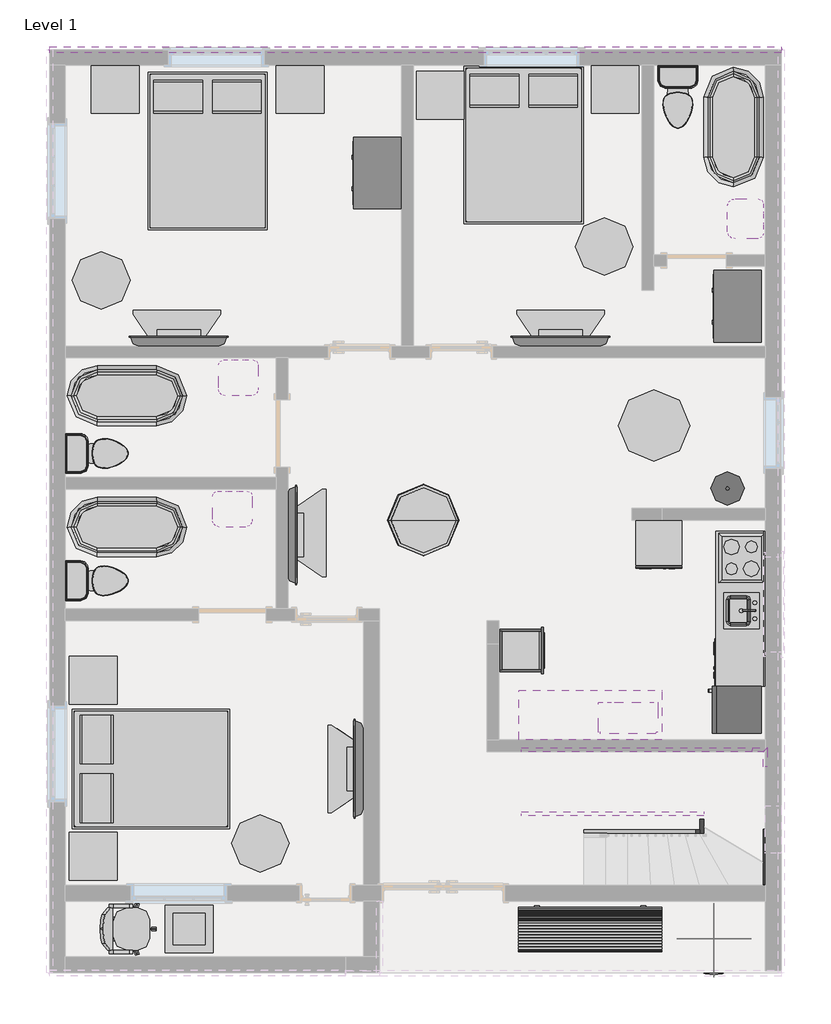
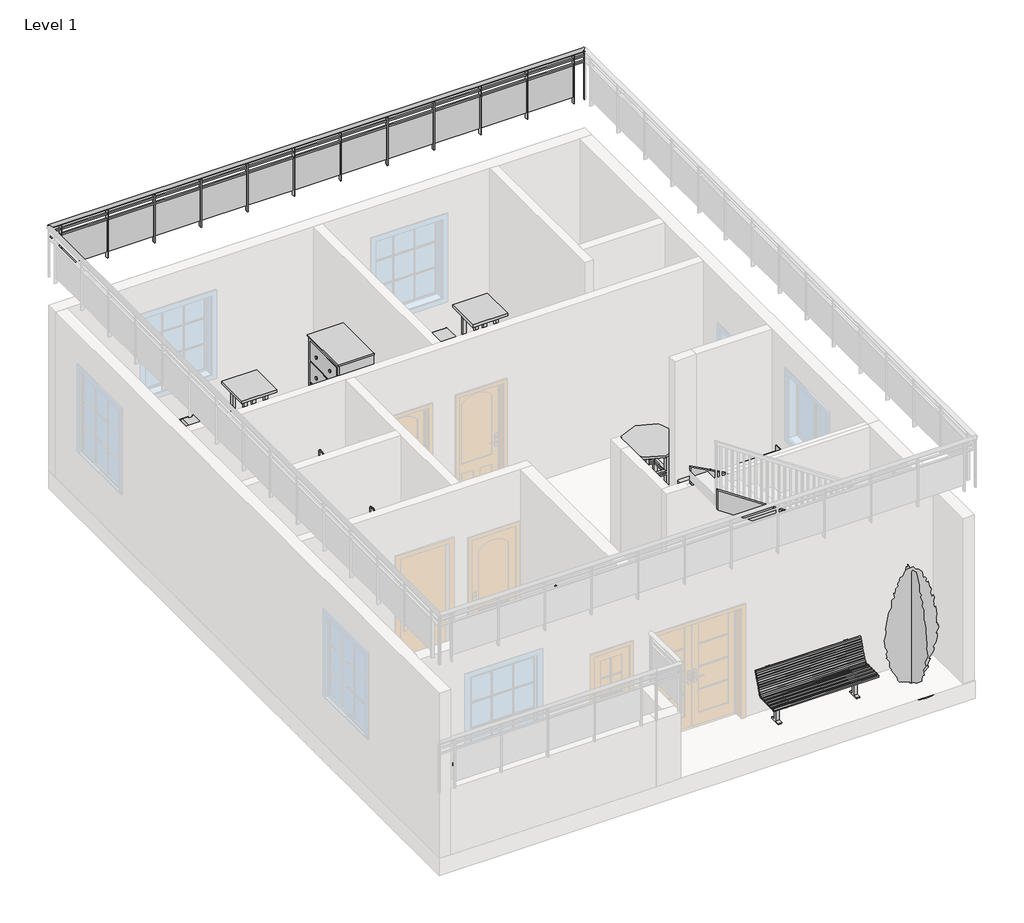
# One storey, part 4 of 4: 28 furniture elements, 11 flow terminals, 10 members, 7 proxies, 2 geographic elements, 1 railing.
"""IFC4 building model written with IfcOpenShell, lengths in millimetres."""

from ifc_helpers import new_model, si_unit, point, frame, origin, place, context, project, spatial, polyline, ellipse_curve, trimmed, outline, extrude, transform, mapped, element, save
from ifc_brep_helpers import plane_surface, extruded_surface, advanced_brep
from components import proxy_a6faaae8, proxy_53e5fb40, proxy_45b28599, kitchenette_medium_kitchenette_medium_844211aa, proxy_8a8d5ab2, proxy_8b8c2dc4, proxy_c523a7b7, flow_terminal_871c2e40, flow_terminal_d49f872f, flow_terminal_62a433f7, toilet_domestic_3d_toilet_domestic_3d_f7549cf7, toilet_domestic_3d_toilet_domestic_3d_183bbd19, flow_terminal_b374fae2, furniture_1d2926bd, chair_executive_chair_executive_8d69e98c, furniture_c6510c7c, furniture_1447f48d, furniture_33655958, furniture_fdf74506, tv_stand_tv_stand_6ce107e5, furniture_b5c51a22, furniture_905aceb5, furniture_b2396e53, furniture_5bc9ed15, furniture_c80d6d9c, geographic_element_235d1464, rpc_tree_conifer_chinese_juniper_7_1b9786cd

model = new_model("IFC4")

# Units and contexts
model_context = context("Model", 3, world=origin())
ifc_project = project(units=[si_unit("LENGTHUNIT", "METRE", prefix="MILLI")], contexts=[model_context])

# Site, building, storey
site = spatial("IfcSite", under=ifc_project)
building = spatial("IfcBuilding", under=site)
storey = spatial("IfcBuildingStorey", under=building, Name="Level 1", Elevation=0.0)

# Proxies
placement = place(None, origin())
proxy_shape = proxy_a6faaae8(model_context)
element("IfcBuildingElementProxy", 1, Name="Cook Top-4 Unit2 : 22\" x 20\"", ObjectType="Cook Top-4 Unit2 : 22\" x 20\"", at=placement, inside=storey, context=model_context, shape_type="MappedRepresentation", body=[
    mapped(proxy_shape, transform((5037.4355823, 3615.7840324, 0.0), x_axis=(0.0, -1.0000000000000002, 0.0), y_axis=(1.0000000000000002, 0.0, 0.0), z_axis=(0.0, 0.0, 1.0))),
])
proxy_2_shape = proxy_53e5fb40(model_context)
element("IfcBuildingElementProxy", 2, Name="Dishwasher : 23\" x 23 11/16\" x 33 1/2\"", ObjectType="Dishwasher : 23\" x 23 11/16\" x 33 1/2\"", at=placement, inside=storey, context=model_context, shape_type="MappedRepresentation", body=[
    mapped(proxy_2_shape, transform((3613.7181138, 3535.0719677, 0.0), x_axis=(1.0000000000000002, 0.0, 0.0), y_axis=(0.0, 1.0000000000000002, 0.0), z_axis=(0.0, 0.0, 1.0))),
])
proxy_3_shape = proxy_45b28599(model_context)
element("IfcBuildingElementProxy", 3, Name="Dishwasher : 24\" x 24\" x 34\"", ObjectType="Dishwasher : 24\" x 24\" x 34\"", at=placement, inside=storey, context=model_context, shape_type="MappedRepresentation", body=[
    mapped(proxy_3_shape, transform((4745.5860175, 2664.6015009, 0.0), x_axis=(0.0, -1.0000000000000002, 0.0), y_axis=(1.0000000000000002, 0.0, 0.0), z_axis=(0.0, 0.0, 1.0))),
])
kitchenette_medium_kitchenette_medium_shape = kitchenette_medium_kitchenette_medium_844211aa(model_context)
element("IfcBuildingElementProxy", 4, Name="Kitchenette - Medium : Kitchenette - Medium", ObjectType="Kitchenette - Medium : Kitchenette - Medium", at=placement, inside=storey, context=model_context, shape_type="MappedRepresentation", body=[
    mapped(kitchenette_medium_kitchenette_medium_shape, transform((5342.2355823, 3291.6217374, 0.0), x_axis=(0.0, -1.0000000000000002, 0.0), y_axis=(1.0000000000000002, 0.0, 0.0), z_axis=(0.0, 0.0, 1.0))),
])
proxy_4_shape = proxy_8a8d5ab2(model_context)
element("IfcBuildingElementProxy", 5, Name="Microwave : 30\" x 16\" x 18\"", ObjectType="Microwave : 30\" x 16\" x 18\"", at=placement, inside=storey, context=model_context, shape_type="MappedRepresentation", body=[
    mapped(proxy_4_shape, transform((4089.9284596, 1218.0035266, 609.6), x_axis=(-1.0000000000000004, 0.0, 0.0), y_axis=(0.0, -1.0000000000000004, 0.0), z_axis=(0.0, 0.0, 1.0))),
])
proxy_5_shape = proxy_8b8c2dc4(model_context)
element("IfcBuildingElementProxy", 6, Name="Oven Double-Built-in : 21 1/2\" x 39 1/4\" x 21\"", ObjectType="Oven Double-Built-in : 21 1/2\" x 39 1/4\" x 21\"", at=placement, inside=storey, context=model_context, shape_type="MappedRepresentation", body=[
    mapped(proxy_5_shape, transform((2359.1014412, 2469.8589597, 0.0), x_axis=(0.0, 1.0000000000000002, 0.0), y_axis=(-1.0000000000000002, 0.0, 0.0), z_axis=(0.0, 0.0, 1.0))),
])
proxy_6_shape = proxy_c523a7b7(model_context)
element("IfcBuildingElementProxy", 7, Name="Refrigerator : 24\" x 25\" LH", ObjectType="Refrigerator : 24\" x 25\" LH", at=placement, inside=storey, context=model_context, shape_type="MappedRepresentation", body=[
    mapped(proxy_6_shape, transform((4991.7866108, 1679.0340324, 0.0), x_axis=(0.0, -1.0000000000000002, 0.0), y_axis=(1.0000000000000002, 0.0, 0.0), z_axis=(0.0, 0.0, 1.0))),
])

# Flow terminals
flow_terminal_shape = flow_terminal_871c2e40(model_context)
element("IfcFlowTerminal", 8, ObjectType="Sink Kitchen-Island : 18\" x 18\"", at=placement, inside=storey, context=model_context, shape_type="MappedRepresentation", body=[
    mapped(flow_terminal_shape, transform((5035.0901812, 2958.373273, -14.4), x_axis=(0.0, -1.0000000000000002, 0.0), y_axis=(1.0000000000000002, 0.0, 0.0), z_axis=(0.0, 0.0, 1.0))),
])
flow_terminal_2_shape = flow_terminal_d49f872f(model_context)
element("IfcFlowTerminal", 9, ObjectType="Sink Vanity-Round : 19\" x 19\"", at=placement, inside=storey, context=model_context, shape_type="MappedRepresentation", body=[
    mapped(flow_terminal_2_shape, transform((4956.2873228, 4587.4155119, 609.6), x_axis=(-1.0000000000000004, 0.0, 0.0), y_axis=(0.0, -1.0000000000000004, 0.0), z_axis=(0.0, 0.0, 1.0))),
])
flow_terminal_3_shape = flow_terminal_62a433f7(model_context)
element("IfcFlowTerminal", 10, ObjectType="Sink Vanity-Square : 20\" x 18\"", at=placement, inside=storey, context=model_context, shape_type="MappedRepresentation", body=[
    mapped(flow_terminal_3_shape, transform((-1404.4536583, 5962.9386313, 914.4), x_axis=(1.0, 0.0, 0.0), y_axis=(0.0, 1.0, 0.0), z_axis=(0.0, 0.0, 1.0))),
])
element("IfcFlowTerminal", 11, ObjectType="Sink Vanity-Square : 20\" x 18\"", at=placement, inside=storey, context=model_context, shape_type="MappedRepresentation", body=[
    mapped(flow_terminal_3_shape, transform((-1480.6536583, 4286.5386313, 914.4), x_axis=(1.0, 0.0, 0.0), y_axis=(0.0, 1.0, 0.0), z_axis=(0.0, 0.0, 1.0))),
])
element("IfcFlowTerminal", 12, ObjectType="Sink Vanity-Square : 20\" x 18\"", at=placement, inside=storey, context=model_context, shape_type="MappedRepresentation", body=[
    mapped(flow_terminal_3_shape, transform((5136.6901812, 7962.173273, 914.4), x_axis=(0.0, -1.0, 0.0), y_axis=(1.0, 0.0, 0.0), z_axis=(0.0, 0.0, 1.0))),
])
toilet_domestic_3d_toilet_domestic_3d_shape = toilet_domestic_3d_toilet_domestic_3d_f7549cf7(model_context)
toilet_domestic_3d_toilet_domestic_3d_2_shape = toilet_domestic_3d_toilet_domestic_3d_183bbd19(model_context)
element("IfcFlowTerminal", 13, ObjectType="Toilet-Domestic-3D : Toilet-Domestic-3D", at=placement, inside=storey, context=model_context, shape_type="MappedRepresentation", body=[
    mapped(toilet_domestic_3d_toilet_domestic_3d_shape, transform((-3103.8683904, 4949.2840324, 0.0), x_axis=(0.0, 1.0000000000000002, 0.0), y_axis=(-1.0000000000000002, 0.0, 0.0), z_axis=(0.0, 0.0, 1.0))),
    mapped(toilet_domestic_3d_toilet_domestic_3d_2_shape, transform((-3103.8683904, 4949.2840324, 0.0), x_axis=(0.0, 1.0000000000000002, 0.0), y_axis=(-1.0000000000000002, 0.0, 0.0), z_axis=(0.0, 0.0, 1.0))),
])
element("IfcFlowTerminal", 14, ObjectType="Toilet-Domestic-3D : Toilet-Domestic-3D", at=placement, inside=storey, context=model_context, shape_type="MappedRepresentation", body=[
    mapped(toilet_domestic_3d_toilet_domestic_3d_shape, transform((-3103.8683904, 3323.6840324, 0.0), x_axis=(0.0, 1.0000000000000002, 0.0), y_axis=(-1.0000000000000002, 0.0, 0.0), z_axis=(0.0, 0.0, 1.0))),
    mapped(toilet_domestic_3d_toilet_domestic_3d_2_shape, transform((-3103.8683904, 3323.6840324, 0.0), x_axis=(0.0, 1.0000000000000002, 0.0), y_axis=(-1.0000000000000002, 0.0, 0.0), z_axis=(0.0, 0.0, 1.0))),
])
element("IfcFlowTerminal", 15, ObjectType="Toilet-Domestic-3D : Toilet-Domestic-3D", at=placement, inside=storey, context=model_context, shape_type="MappedRepresentation", body=[
    mapped(toilet_domestic_3d_toilet_domestic_3d_shape, transform((4224.6355823, 9407.5880051, 0.0), x_axis=(1.0, 0.0, 0.0), y_axis=(0.0, 1.0, 0.0), z_axis=(0.0, 0.0, 1.0))),
    mapped(toilet_domestic_3d_toilet_domestic_3d_2_shape, transform((4224.6355823, 9407.5880051, 0.0), x_axis=(1.0, 0.0, 0.0), y_axis=(0.0, 1.0, 0.0), z_axis=(0.0, 0.0, 1.0))),
])
flow_terminal_4_shape = flow_terminal_b374fae2(model_context)
element("IfcFlowTerminal", 16, ObjectType="Tub-Free Standing-3D : 30\" x 60\"", at=placement, inside=storey, context=model_context, shape_type="MappedRepresentation", body=[
    mapped(flow_terminal_4_shape, transform((-2811.1644177, 4009.4840324, 0.0), x_axis=(0.0, 1.0000000000000002, 0.0), y_axis=(-1.0000000000000002, 0.0, 0.0), z_axis=(0.0, 0.0, 1.0))),
])
element("IfcFlowTerminal", 17, ObjectType="Tub-Free Standing-3D : 30\" x 60\"", at=placement, inside=storey, context=model_context, shape_type="MappedRepresentation", body=[
    mapped(flow_terminal_4_shape, transform((-2811.1644177, 5685.8840324, 0.0), x_axis=(0.0, 1.0000000000000002, 0.0), y_axis=(-1.0000000000000002, 0.0, 0.0), z_axis=(0.0, 0.0, 1.0))),
])
element("IfcFlowTerminal", 18, ObjectType="Tub-Free Standing-3D : 30\" x 60\"", at=placement, inside=storey, context=model_context, shape_type="MappedRepresentation", body=[
    mapped(flow_terminal_4_shape, transform((4935.8355823, 9114.8840324, 0.0), x_axis=(1.0000000000000007, 0.0, 0.0), y_axis=(0.0, 1.0000000000000007, 0.0), z_axis=(0.0, 0.0, 1.0))),
])

# Furniture
furniture_shape = furniture_1d2926bd(model_context)
element("IfcFurniture", 19, ObjectType="Bed-Box : Queen 60\" x 79\"", at=placement, inside=storey, context=model_context, shape_type="MappedRepresentation", body=[
    mapped(furniture_shape, transform((-2740.7939259, 584.2315734, 0.0), x_axis=(0.0, 1.0000000000000002, 0.0), y_axis=(-1.0000000000000002, 0.0, 0.0), z_axis=(0.0, 0.0, 1.0))),
])
element("IfcFurniture", 20, ObjectType="Bed-Box : Queen 60\" x 79\"", at=placement, inside=storey, context=model_context, shape_type="MappedRepresentation", body=[
    mapped(furniture_shape, transform((-2121.6168767, 9044.5135406, 0.0), x_axis=(1.0000000000000002, 0.0, 0.0), y_axis=(0.0, 1.0000000000000002, 0.0), z_axis=(0.0, 0.0, 1.0))),
])
element("IfcFurniture", 21, ObjectType="Bed-Box : Queen 60\" x 79\"", at=placement, inside=storey, context=model_context, shape_type="MappedRepresentation", body=[
    mapped(furniture_shape, transform((1916.9831233, 9120.7135406, 0.0), x_axis=(1.0, 0.0, 0.0), y_axis=(0.0, 1.0, 0.0), z_axis=(0.0, 0.0, 1.0))),
])
chair_executive_chair_executive_shape = chair_executive_chair_executive_8d69e98c(model_context)
element("IfcFurniture", 22, ObjectType="Chair-Executive : Chair-Executive", at=placement, inside=storey, context=model_context, shape_type="MappedRepresentation", body=[
    mapped(chair_executive_chair_executive_shape, transform((-2804.7103194, -980.3251479, 0.0), x_axis=(0.0, -1.0000000000000004, 0.0), y_axis=(1.0000000000000004, 0.0, 0.0), z_axis=(0.0, 0.0, 1.0))),
])
furniture_2_shape = furniture_c6510c7c(model_context)
element("IfcFurniture", 23, ObjectType="Counter Top w Sink Hole : 24\" Depth", at=placement, inside=storey, context=model_context, shape_type="MappedRepresentation", body=[
    mapped(furniture_2_shape, transform((5342.2355823, 2758.2217374, -14.4), x_axis=(0.0, -1.0000000000000002, 0.0), y_axis=(1.0000000000000002, 0.0, 0.0), z_axis=(0.0, 0.0, 1.0))),
])
furniture_3_shape = furniture_1447f48d(model_context)
element("IfcFurniture", 24, ObjectType="Counter Top w Sink Hole : 24\" Depth", at=placement, inside=storey, context=model_context, shape_type="MappedRepresentation", body=[
    mapped(furniture_3_shape, transform((3393.0978774, 1926.6840324, 609.6), x_axis=(1.0, 0.0, 0.0), y_axis=(0.0, 1.0, 0.0), z_axis=(0.0, 0.0, 1.0))),
])
furniture_4_shape = furniture_33655958(model_context)
element("IfcFurniture", 25, ObjectType="Dresser : 48\" x 72\" x 24\"", at=placement, inside=storey, context=model_context, shape_type="MappedRepresentation", body=[
    mapped(furniture_4_shape, transform((5349.7985364, 6559.6907726, 0.0), x_axis=(0.0, -1.0000000000000007, 0.0), y_axis=(1.0000000000000007, 0.0, 0.0), z_axis=(0.0, 0.0, 1.0))),
])
element("IfcFurniture", 26, ObjectType="Dresser : 48\" x 72\" x 24\"", at=placement, inside=storey, context=model_context, shape_type="MappedRepresentation", body=[
    mapped(furniture_4_shape, transform((752.3985364, 8261.4907726, 0.0), x_axis=(0.0, -1.0000000000000007, 0.0), y_axis=(1.0000000000000007, 0.0, 0.0), z_axis=(0.0, 0.0, 1.0))),
])
furniture_5_shape = furniture_fdf74506(model_context)
element("IfcFurniture", 27, ObjectType="TV - Flat Screen : 50\"", at=placement, inside=storey, context=model_context, shape_type="MappedRepresentation", body=[
    mapped(furniture_5_shape, transform((152.8969586, 919.4395183, 914.4), x_axis=(0.0, -1.0, 0.0), y_axis=(1.0, 0.0, 0.0), z_axis=(0.0, 0.0, 1.0))),
])
element("IfcFurniture", 28, ObjectType="TV - Flat Screen : 50\"", at=placement, inside=storey, context=model_context, shape_type="MappedRepresentation", body=[
    mapped(furniture_5_shape, transform((-2154.7089319, 6379.4226561, 914.4), x_axis=(-1.0, 0.0, 0.0), y_axis=(0.0, -1.0, 0.0), z_axis=(0.0, 0.0, 1.0))),
])
element("IfcFurniture", 29, ObjectType="TV - Flat Screen : 50\"", at=placement, inside=storey, context=model_context, shape_type="MappedRepresentation", body=[
    mapped(furniture_5_shape, transform((2722.0910681, 6379.4226561, 914.4), x_axis=(-1.0, 0.0, 0.0), y_axis=(0.0, -1.0, 0.0), z_axis=(0.0, 0.0, 1.0))),
])
element("IfcFurniture", 30, ObjectType="TV - Flat Screen : 50\"", at=placement, inside=storey, context=model_context, shape_type="MappedRepresentation", body=[
    mapped(furniture_5_shape, transform((-710.8646081, 3912.7153249, 914.4), x_axis=(0.0, 1.0000000000000004, 0.0), y_axis=(-1.0000000000000004, 0.0, 0.0), z_axis=(0.0, 0.0, 1.0))),
])
tv_stand_tv_stand_shape = tv_stand_tv_stand_6ce107e5(model_context)
element("IfcFurniture", 31, ObjectType="TV Stand : TV Stand", at=placement, inside=storey, context=model_context, shape_type="MappedRepresentation", body=[
    mapped(tv_stand_tv_stand_shape, transform((-2050.9764157, 6320.8840324, 0.0), x_axis=(-0.9999999999999998, 0.0, 0.0), y_axis=(0.0, -0.9999999999999998, 0.0), z_axis=(0.0, 0.0, 1.0))),
])
element("IfcFurniture", 32, ObjectType="TV Stand : TV Stand", at=placement, inside=storey, context=model_context, shape_type="MappedRepresentation", body=[
    mapped(tv_stand_tv_stand_shape, transform((2851.2235843, 6320.8840324, 0.0), x_axis=(-1.0, 0.0, 0.0), y_axis=(0.0, -1.0, 0.0), z_axis=(0.0, 0.0, 1.0))),
])
element("IfcFurniture", 33, ObjectType="TV Stand : TV Stand", at=placement, inside=storey, context=model_context, shape_type="MappedRepresentation", body=[
    mapped(tv_stand_tv_stand_shape, transform((211.4355823, 1048.5720345, 0.0), x_axis=(0.0, -1.0, 0.0), y_axis=(1.0, 0.0, 0.0), z_axis=(0.0, 0.0, 1.0))),
])
element("IfcFurniture", 34, ObjectType="TV Stand : TV Stand", at=placement, inside=storey, context=model_context, shape_type="MappedRepresentation", body=[
    mapped(tv_stand_tv_stand_shape, transform((-725.683901, 3808.7141968, 0.0), x_axis=(0.0, 1.0000000000000004, 0.0), y_axis=(-1.0000000000000004, 0.0, 0.0), z_axis=(0.0, 0.0, 1.0))),
])
furniture_6_shape = furniture_b5c51a22(model_context)
element("IfcFurniture", 35, ObjectType="Table-Coffee : 24\" x 24\" x 24\"", at=placement, inside=storey, context=model_context, shape_type="MappedRepresentation", body=[
    mapped(furniture_6_shape, transform((-2035.6801844, -1216.5270454, 0.0), x_axis=(1.0, 0.0, 0.0), y_axis=(0.0, 1.0, 0.0), z_axis=(0.0, 0.0, 1.0))),
])
furniture_7_shape = furniture_905aceb5(model_context)
element("IfcFurniture", 36, ObjectType="Table-Dining Round w Chairs : 36\" Diameter", at=placement, inside=storey, context=model_context, shape_type="MappedRepresentation", body=[
    mapped(furniture_7_shape, transform((3816.1536151, 5489.762721, 0.0), x_axis=(1.0, 0.0, 0.0), y_axis=(0.0, 1.0, 0.0), z_axis=(0.0, 0.0, 1.0))),
])
furniture_8_shape = furniture_b2396e53(model_context)
element("IfcFurniture", 37, ObjectType="Table-Ellipse : 72\" x 36\"", at=placement, inside=storey, context=model_context, shape_type="MappedRepresentation", body=[
    mapped(furniture_8_shape, transform((-1109.3644177, -29.1159676, 0.0), x_axis=(1.0, 0.0, 0.0), y_axis=(0.0, 1.0, 0.0), z_axis=(0.0, 0.0, 1.0))),
])
element("IfcFurniture", 38, ObjectType="Table-Ellipse : 72\" x 36\"", at=placement, inside=storey, context=model_context, shape_type="MappedRepresentation", body=[
    mapped(furniture_8_shape, transform((-3141.3644177, 7159.0840324, 0.0), x_axis=(0.0, 1.0000000000000002, 0.0), y_axis=(-1.0000000000000002, 0.0, 0.0), z_axis=(0.0, 0.0, 1.0))),
])
element("IfcFurniture", 39, ObjectType="Table-Ellipse : 72\" x 36\"", at=placement, inside=storey, context=model_context, shape_type="MappedRepresentation", body=[
    mapped(furniture_8_shape, transform((3284.8355823, 7590.8840324, 0.0), x_axis=(0.0, 1.0000000000000002, 0.0), y_axis=(-1.0000000000000002, 0.0, 0.0), z_axis=(0.0, 0.0, 1.0))),
])
furniture_9_shape = furniture_5bc9ed15(model_context)
element("IfcFurniture", 40, ObjectType="Table-Night Stand : 24\" x 24\" x 30\"", at=placement, inside=storey, context=model_context, shape_type="MappedRepresentation", body=[
    mapped(furniture_9_shape, transform((-3272.098048, 9292.6840324, 0.0), x_axis=(1.0, 0.0, 0.0), y_axis=(0.0, 1.0, 0.0), z_axis=(0.0, 0.0, 1.0))),
])
element("IfcFurniture", 41, ObjectType="Table-Night Stand : 24\" x 24\" x 30\"", at=placement, inside=storey, context=model_context, shape_type="MappedRepresentation", body=[
    mapped(furniture_9_shape, transform((-909.898048, 9292.6840324, 0.0), x_axis=(1.0, 0.0, 0.0), y_axis=(0.0, 1.0, 0.0), z_axis=(0.0, 0.0, 1.0))),
])
element("IfcFurniture", 42, ObjectType="Table-Night Stand : 24\" x 24\" x 30\"", at=placement, inside=storey, context=model_context, shape_type="MappedRepresentation", body=[
    mapped(furniture_9_shape, transform((880.801952, 9216.4840324, 0.0), x_axis=(1.0, 0.0, 0.0), y_axis=(0.0, 1.0, 0.0), z_axis=(0.0, 0.0, 1.0))),
])
element("IfcFurniture", 43, ObjectType="Table-Night Stand : 24\" x 24\" x 30\"", at=placement, inside=storey, context=model_context, shape_type="MappedRepresentation", body=[
    mapped(furniture_9_shape, transform((3116.001952, 9292.6840324, 0.0), x_axis=(1.0, 0.0, 0.0), y_axis=(0.0, 1.0, 0.0), z_axis=(0.0, 0.0, 1.0))),
])
element("IfcFurniture", 44, ObjectType="Table-Night Stand : 24\" x 24\" x 30\"", at=placement, inside=storey, context=model_context, shape_type="MappedRepresentation", body=[
    mapped(furniture_9_shape, transform((-3551.498048, 1748.8840324, 0.0), x_axis=(1.0, 0.0, 0.0), y_axis=(0.0, 1.0, 0.0), z_axis=(0.0, 0.0, 1.0))),
])
element("IfcFurniture", 45, ObjectType="Table-Night Stand : 24\" x 24\" x 30\"", at=placement, inside=storey, context=model_context, shape_type="MappedRepresentation", body=[
    mapped(furniture_9_shape, transform((-3551.498048, -499.0159676, 0.0), x_axis=(1.0, 0.0, 0.0), y_axis=(0.0, 1.0, 0.0), z_axis=(0.0, 0.0, 1.0))),
])
furniture_10_shape = furniture_c80d6d9c(model_context)
element("IfcFurniture", 46, ObjectType="Table-Round : 36\" Diameter", at=placement, inside=storey, context=model_context, shape_type="MappedRepresentation", body=[
    mapped(furniture_10_shape, transform((973.4355823, 4098.3840324, 0.0), x_axis=(1.0, 0.0, 0.0), y_axis=(0.0, 1.0, 0.0), z_axis=(0.0, 0.0, 1.0))),
])

# Geographic elements
geographic_element_shape = geographic_element_235d1464(model_context)
element("IfcGeographicElement", 47, ObjectType="Park Bench : 72\"", at=placement, inside=storey, context=model_context, shape_type="MappedRepresentation", body=[
    mapped(geographic_element_shape, transform((3103.3038904, -1095.9159676, 0.0), x_axis=(1.0, 0.0, 0.0), y_axis=(0.0, 1.0, 0.0), z_axis=(0.0, 0.0, 1.0))),
])
rpc_tree_conifer_chinese_juniper_7_shape = rpc_tree_conifer_chinese_juniper_7_1b9786cd(model_context)
element("IfcGeographicElement", 48, ObjectType="RPC Tree - Conifer : Chinese Juniper - 7'", at=placement, inside=storey, context=model_context, shape_type="MappedRepresentation", body=[
    mapped(rpc_tree_conifer_chinese_juniper_7_shape, transform((4681.6389112, -1248.3159676, 0.0), x_axis=(1.0, 0.0, 0.0), y_axis=(0.0, 1.0, 0.0), z_axis=(0.0, 0.0, 1.0))),
])

# Members
element("IfcMember", 49, ObjectType="Stringer - 2\" Width", at=placement, inside=storey, context=model_context, shape_type="SweptSolid", body=[
    extrude(outline(polyline([(193.875111, 3027.1038904), (0.0, 3027.1038904), (0.0, 3280.7417408), (866.2306092, 4504.0355823), (1239.7100492, 4504.0355823), (193.875111, 3027.1038904)])), frame((0.0, 97.8840324, 0.0), z_axis=(0.0, 1.0, 0.0), x_axis=(0.0, 0.0, 1.0)), (0.0, 0.0, 1.0), 50.8),
])
element("IfcMember", 50, ObjectType="Stringer - 2\" Width", at=placement, inside=storey, context=model_context, shape_type="SweptSolid", body=[
    extrude(outline(polyline([(97.8840324, 902.2027636), (97.8840324, 1511.3383296), (285.7663347, 1885.6140258), (326.4840324, 1885.6140258), (326.4840324, 1287.3328071), (133.1529667, 902.2027636), (97.8840324, 902.2027636)])), frame((4504.0355823, 0.0, 0.0), z_axis=(1.0, 0.0, 0.0), x_axis=(0.0, 1.0, 0.0)), (0.0, 0.0, 1.0), 50.8),
])
element("IfcMember", 51, ObjectType="Stringer - 2\" Width", at=placement, inside=storey, context=model_context, shape_type="SweptSolid", body=[
    extrude(outline(polyline([(1518.0253455, 4554.8355823), (1885.6140258, 4554.8355823), (3455.1530234, 2226.5502663), (3087.5643431, 2226.5502663), (1518.0253455, 4554.8355823)])), frame((0.0, 326.4840324, 0.0), z_axis=(0.0, 1.0, 0.0), x_axis=(0.0, 0.0, 1.0)), (0.0, 0.0, 1.0), 50.8),
])
element("IfcMember", 52, ObjectType="Stringer - 2\" Width", at=placement, inside=storey, context=model_context, shape_type="SweptSolid", body=[
    extrude(outline(polyline([(228.7465266, 3027.1038904), (0.0, 3027.1038904), (0.0, 3247.9011968), (961.7958595, 5098.1688903), (1305.3160136, 5098.1688903), (228.7465266, 3027.1038904)])), frame((0.0, -714.9159676, 0.0), z_axis=(0.0, 1.0, 0.0), x_axis=(0.0, 0.0, 1.0)), (0.0, 0.0, 1.0), 50.8),
])
element("IfcMember", 53, ObjectType="Stringer - 2\" Width", at=placement, inside=storey, context=model_context, shape_type="SweptSolid", body=[
    extrude(outline(polyline([(5098.1688903, -714.9159676), (5098.1688903, -664.1159676), (5316.8355823, -664.1159676), (5367.6355823, -714.9159676), (5098.1688903, -714.9159676)])), frame((0.0, 0.0, 961.7958595), z_axis=(0.0, 0.0, 1.0), x_axis=(1.0, 0.0, 0.0)), (0.0, 0.0, 1.0), 343.5201541),
])
element("IfcMember", 54, ObjectType="Stringer - 2\" Width", at=placement, inside=storey, context=model_context, shape_type="SweptSolid", body=[
    extrude(outline(polyline([(5367.6355823, -714.9159676), (5316.8355823, -664.1159676), (5316.8355823, -554.627196), (5367.6355823, -554.627196), (5367.6355823, -714.9159676)])), frame((0.0, 0.0, 961.7958595), z_axis=(0.0, 0.0, 1.0), x_axis=(1.0, 0.0, 0.0)), (0.0, 0.0, 1.0), 343.5201541),
])
element("IfcMember", 55, ObjectType="Stringer - 2\" Width", at=placement, inside=storey, context=model_context, shape_type="SweptSolid", body=[
    extrude(outline(polyline([(-554.627196, 961.7958595), (-554.627196, 1305.3160136), (947.5106454, 1813.3160136), (947.5106454, 1469.7958595), (-554.627196, 961.7958595)])), frame((5316.8355823, 0.0, 0.0), z_axis=(1.0, 0.0, 0.0), x_axis=(0.0, 1.0, 0.0)), (0.0, 0.0, 1.0), 50.8),
])
element("IfcMember", 56, ObjectType="Stringer - 2\" Width", at=placement, inside=storey, context=model_context, shape_type="SweptSolid", body=[
    extrude(outline(polyline([(5367.6355823, 947.5106454), (5316.8355823, 947.5106454), (5316.8355823, 1139.2840324), (5367.6355823, 1190.0840324), (5367.6355823, 947.5106454)])), frame((0.0, 0.0, 1480.0963717), z_axis=(0.0, 0.0, 1.0), x_axis=(1.0, 0.0, 0.0)), (0.0, 0.0, 1.0), 321.7580709),
])
element("IfcMember", 57, ObjectType="Stringer - 2\" Width", at=placement, inside=storey, context=model_context, shape_type="SweptSolid", body=[
    extrude(outline(polyline([(5367.6355823, 1190.0840324), (5316.8355823, 1139.2840324), (5177.8533218, 1139.2840324), (5177.8533218, 1190.0840324), (5367.6355823, 1190.0840324)])), frame((0.0, 0.0, 1480.0963717), z_axis=(0.0, 0.0, 1.0), x_axis=(1.0, 0.0, 0.0)), (0.0, 0.0, 1.0), 321.7580709),
])
element("IfcMember", 58, ObjectType="Stringer - 2\" Width", at=placement, inside=storey, context=model_context, shape_type="SweptSolid", body=[
    extrude(outline(polyline([(1480.0963717, 5177.8533218), (1801.8544427, 5177.8533218), (3391.6983765, 2226.5502663), (3069.9403056, 2226.5502663), (1480.0963717, 5177.8533218)])), frame((0.0, 1139.2840324, 0.0), z_axis=(0.0, 1.0, 0.0), x_axis=(0.0, 0.0, 1.0)), (0.0, 0.0, 1.0), 50.8),
])

# Railing
element("IfcRailing", 59, ObjectType="Glass Panel - Bottom Fill", at=placement, inside=storey, context=model_context, shape_type="SolidModel", body=[
    advanced_brep(
    [(-3801.7644177, 10143.5840324, 4495.8), (-3801.7644177, 10067.3840324, 4495.8), (5545.4355823, 10143.5840324, 4495.8), (5545.4355823, 10067.3840324, 4495.8)],
    [
        (0, 1, ellipse_curve(frame((-3801.7644177, 10105.4840324, 4495.8), z_axis=(-1.0, 0.0, 0.0), x_axis=(0.0, -1.0, 0.0)), 38.1, 28.575)),
        (1, 0, ellipse_curve(frame((-3801.7644177, 10105.4840324, 4495.8), z_axis=(-1.0, 0.0, 0.0), x_axis=(0.0, -1.0, 0.0)), 38.1, 28.575)),
        (2, 3, ellipse_curve(frame((5545.4355823, 10105.4840324, 4495.8), z_axis=(1.0, 0.0, 0.0), x_axis=(0.0, -1.0, 0.0)), 38.1, 28.575)),
        (3, 2, ellipse_curve(frame((5545.4355823, 10105.4840324, 4495.8), z_axis=(1.0, 0.0, 0.0), x_axis=(0.0, -1.0, 0.0)), 38.1, 28.575)),
        (0, 2),
        (3, 1),
    ],
    [
        plane_surface(frame((-3801.7644177, 10105.4840324, 4495.8), z_axis=(-1.0, 0.0, 0.0), x_axis=(0.0, 1.0, 0.0))),
        plane_surface(frame((5545.4355823, 10105.4840324, 4495.8), z_axis=(1.0, 0.0, 0.0), x_axis=(0.0, 1.0, 0.0))),
        extruded_surface(trimmed(ellipse_curve(frame((5545.4355823, 10105.4840324, 4495.8), z_axis=(-1.0, 0.0, 0.0), x_axis=(0.0, -1.0, 0.0)), 38.1, 28.575), [point((5545.4355823, 10143.5840324, 4495.8))], [point((5545.4355823, 10067.3840324, 4495.8))], True, "CARTESIAN"), (-9347.2, 0.0, 0.0), 9347.2),
        extruded_surface(trimmed(ellipse_curve(frame((5545.4355823, 10105.4840324, 4495.8), z_axis=(-1.0, 0.0, 0.0), x_axis=(0.0, -1.0, 0.0)), 38.1, 28.575), [point((5545.4355823, 10067.3840324, 4495.8))], [point((5545.4355823, 10143.5840324, 4495.8))], True, "CARTESIAN"), (-9347.2, 0.0, 0.0), 9347.2),
    ],
    [
        (0, [[1, 2]]),
        (1, [[3, 4]]),
        (2, [[-1, 5, -4, 6]]),
        (3, [[-2, -6, -3, -5]]),
    ],
),
    extrude(outline(polyline([(-3801.7644177, 10092.7840324), (-3801.7644177, 10118.1840324), (5545.4355823, 10118.1840324), (5545.4355823, 10092.7840324), (-3801.7644177, 10092.7840324)])), frame((0.0, 0.0, 4381.5), z_axis=(0.0, 0.0, 1.0), x_axis=(1.0, 0.0, 0.0)), (0.0, 0.0, 1.0), 25.4),
    extrude(outline(polyline([(-3801.7644177, 10092.7840324), (-3801.7644177, 10118.1840324), (5545.4355823, 10118.1840324), (5545.4355823, 10092.7840324), (-3801.7644177, 10092.7840324)])), frame((0.0, 0.0, 4279.9), z_axis=(0.0, 0.0, 1.0), x_axis=(1.0, 0.0, 0.0)), (0.0, 0.0, 1.0), 25.4),
    extrude(outline(polyline([(5335.8855823, 10080.0840324), (5335.8855823, 10130.8840324), (5348.5855823, 10130.8840324), (5348.5855823, 10080.0840324), (5335.8855823, 10080.0840324)])), frame((0.0, 0.0, 3581.4), z_axis=(0.0, 0.0, 1.0), x_axis=(1.0, 0.0, 0.0)), (0.0, 0.0, 1.0), 885.6788223),
    extrude(outline(polyline([(4529.4355823, 10112.0191894), (5342.2355823, 10112.0191894), (5342.2355823, 10105.6691894), (4529.4355823, 10105.6691894), (4529.4355823, 10112.0191894)])), frame((0.0, 0.0, 3683.0), z_axis=(0.0, 0.0, 1.0), x_axis=(1.0, 0.0, 0.0)), (0.0, 0.0, 1.0), 596.9),
    extrude(outline(polyline([(4523.0855823, 10080.0840324), (4523.0855823, 10130.8840324), (4535.7855823, 10130.8840324), (4535.7855823, 10080.0840324), (4523.0855823, 10080.0840324)])), frame((0.0, 0.0, 3581.4), z_axis=(0.0, 0.0, 1.0), x_axis=(1.0, 0.0, 0.0)), (0.0, 0.0, 1.0), 885.6788223),
    extrude(outline(polyline([(3716.6355823, 10112.0191894), (4529.4355823, 10112.0191894), (4529.4355823, 10105.6691894), (3716.6355823, 10105.6691894), (3716.6355823, 10112.0191894)])), frame((0.0, 0.0, 3683.0), z_axis=(0.0, 0.0, 1.0), x_axis=(1.0, 0.0, 0.0)), (0.0, 0.0, 1.0), 596.9),
    extrude(outline(polyline([(3710.2855823, 10080.0840324), (3710.2855823, 10130.8840324), (3722.9855823, 10130.8840324), (3722.9855823, 10080.0840324), (3710.2855823, 10080.0840324)])), frame((0.0, 0.0, 3581.4), z_axis=(0.0, 0.0, 1.0), x_axis=(1.0, 0.0, 0.0)), (0.0, 0.0, 1.0), 885.6788223),
    extrude(outline(polyline([(2903.8355823, 10112.0191894), (3716.6355823, 10112.0191894), (3716.6355823, 10105.6691894), (2903.8355823, 10105.6691894), (2903.8355823, 10112.0191894)])), frame((0.0, 0.0, 3683.0), z_axis=(0.0, 0.0, 1.0), x_axis=(1.0, 0.0, 0.0)), (0.0, 0.0, 1.0), 596.9),
    extrude(outline(polyline([(2897.4855823, 10080.0840324), (2897.4855823, 10130.8840324), (2910.1855823, 10130.8840324), (2910.1855823, 10080.0840324), (2897.4855823, 10080.0840324)])), frame((0.0, 0.0, 3581.4), z_axis=(0.0, 0.0, 1.0), x_axis=(1.0, 0.0, 0.0)), (0.0, 0.0, 1.0), 885.6788223),
    extrude(outline(polyline([(2091.0355823, 10112.0191894), (2903.8355823, 10112.0191894), (2903.8355823, 10105.6691894), (2091.0355823, 10105.6691894), (2091.0355823, 10112.0191894)])), frame((0.0, 0.0, 3683.0), z_axis=(0.0, 0.0, 1.0), x_axis=(1.0, 0.0, 0.0)), (0.0, 0.0, 1.0), 596.9),
    extrude(outline(polyline([(2084.6855823, 10080.0840324), (2084.6855823, 10130.8840324), (2097.3855823, 10130.8840324), (2097.3855823, 10080.0840324), (2084.6855823, 10080.0840324)])), frame((0.0, 0.0, 3581.4), z_axis=(0.0, 0.0, 1.0), x_axis=(1.0, 0.0, 0.0)), (0.0, 0.0, 1.0), 885.6788223),
    extrude(outline(polyline([(1278.2355823, 10112.0191894), (2091.0355823, 10112.0191894), (2091.0355823, 10105.6691894), (1278.2355823, 10105.6691894), (1278.2355823, 10112.0191894)])), frame((0.0, 0.0, 3683.0), z_axis=(0.0, 0.0, 1.0), x_axis=(1.0, 0.0, 0.0)), (0.0, 0.0, 1.0), 596.9),
    extrude(outline(polyline([(1271.8855823, 10080.0840324), (1271.8855823, 10130.8840324), (1284.5855823, 10130.8840324), (1284.5855823, 10080.0840324), (1271.8855823, 10080.0840324)])), frame((0.0, 0.0, 3581.4), z_axis=(0.0, 0.0, 1.0), x_axis=(1.0, 0.0, 0.0)), (0.0, 0.0, 1.0), 885.6788223),
    extrude(outline(polyline([(465.4355823, 10112.0191894), (1278.2355823, 10112.0191894), (1278.2355823, 10105.6691894), (465.4355823, 10105.6691894), (465.4355823, 10112.0191894)])), frame((0.0, 0.0, 3683.0), z_axis=(0.0, 0.0, 1.0), x_axis=(1.0, 0.0, 0.0)), (0.0, 0.0, 1.0), 596.9),
    extrude(outline(polyline([(459.0855823, 10080.0840324), (459.0855823, 10130.8840324), (471.7855823, 10130.8840324), (471.7855823, 10080.0840324), (459.0855823, 10080.0840324)])), frame((0.0, 0.0, 3581.4), z_axis=(0.0, 0.0, 1.0), x_axis=(1.0, 0.0, 0.0)), (0.0, 0.0, 1.0), 885.6788223),
    extrude(outline(polyline([(-347.3644177, 10112.0191894), (465.4355823, 10112.0191894), (465.4355823, 10105.6691894), (-347.3644177, 10105.6691894), (-347.3644177, 10112.0191894)])), frame((0.0, 0.0, 3683.0), z_axis=(0.0, 0.0, 1.0), x_axis=(1.0, 0.0, 0.0)), (0.0, 0.0, 1.0), 596.9),
    extrude(outline(polyline([(-353.7144177, 10080.0840324), (-353.7144177, 10130.8840324), (-341.0144177, 10130.8840324), (-341.0144177, 10080.0840324), (-353.7144177, 10080.0840324)])), frame((0.0, 0.0, 3581.4), z_axis=(0.0, 0.0, 1.0), x_axis=(1.0, 0.0, 0.0)), (0.0, 0.0, 1.0), 885.6788223),
    extrude(outline(polyline([(-1160.1644177, 10112.0191894), (-347.3644177, 10112.0191894), (-347.3644177, 10105.6691894), (-1160.1644177, 10105.6691894), (-1160.1644177, 10112.0191894)])), frame((0.0, 0.0, 3683.0), z_axis=(0.0, 0.0, 1.0), x_axis=(1.0, 0.0, 0.0)), (0.0, 0.0, 1.0), 596.9),
    extrude(outline(polyline([(-1166.5144177, 10080.0840324), (-1166.5144177, 10130.8840324), (-1153.8144177, 10130.8840324), (-1153.8144177, 10080.0840324), (-1166.5144177, 10080.0840324)])), frame((0.0, 0.0, 3581.4), z_axis=(0.0, 0.0, 1.0), x_axis=(1.0, 0.0, 0.0)), (0.0, 0.0, 1.0), 885.6788223),
    extrude(outline(polyline([(-1972.9644177, 10112.0191894), (-1160.1644177, 10112.0191894), (-1160.1644177, 10105.6691894), (-1972.9644177, 10105.6691894), (-1972.9644177, 10112.0191894)])), frame((0.0, 0.0, 3683.0), z_axis=(0.0, 0.0, 1.0), x_axis=(1.0, 0.0, 0.0)), (0.0, 0.0, 1.0), 596.9),
    extrude(outline(polyline([(-1979.3144177, 10080.0840324), (-1979.3144177, 10130.8840324), (-1966.6144177, 10130.8840324), (-1966.6144177, 10080.0840324), (-1979.3144177, 10080.0840324)])), frame((0.0, 0.0, 3581.4), z_axis=(0.0, 0.0, 1.0), x_axis=(1.0, 0.0, 0.0)), (0.0, 0.0, 1.0), 885.6788223),
    extrude(outline(polyline([(-2785.7644177, 10112.0191894), (-1972.9644177, 10112.0191894), (-1972.9644177, 10105.6691894), (-2785.7644177, 10105.6691894), (-2785.7644177, 10112.0191894)])), frame((0.0, 0.0, 3683.0), z_axis=(0.0, 0.0, 1.0), x_axis=(1.0, 0.0, 0.0)), (0.0, 0.0, 1.0), 596.9),
    extrude(outline(polyline([(-2792.1144177, 10080.0840324), (-2792.1144177, 10130.8840324), (-2779.4144177, 10130.8840324), (-2779.4144177, 10080.0840324), (-2792.1144177, 10080.0840324)])), frame((0.0, 0.0, 3581.4), z_axis=(0.0, 0.0, 1.0), x_axis=(1.0, 0.0, 0.0)), (0.0, 0.0, 1.0), 885.6788223),
    extrude(outline(polyline([(-3598.5644177, 10112.0191894), (-2785.7644177, 10112.0191894), (-2785.7644177, 10105.6691894), (-3598.5644177, 10105.6691894), (-3598.5644177, 10112.0191894)])), frame((0.0, 0.0, 3683.0), z_axis=(0.0, 0.0, 1.0), x_axis=(1.0, 0.0, 0.0)), (0.0, 0.0, 1.0), 596.9),
    extrude(outline(polyline([(-3604.9144177, 10080.0840324), (-3604.9144177, 10130.8840324), (-3592.2144177, 10130.8840324), (-3592.2144177, 10080.0840324), (-3604.9144177, 10080.0840324)])), frame((0.0, 0.0, 3581.4), z_axis=(0.0, 0.0, 1.0), x_axis=(1.0, 0.0, 0.0)), (0.0, 0.0, 1.0), 885.6788223),
    extrude(outline(polyline([(5532.7355823, 10095.9590324), (5532.7355823, 10115.0090324), (5551.7855823, 10115.0090324), (5551.7855823, 10095.9590324), (5532.7355823, 10095.9590324)])), frame((0.0, 0.0, 3581.4), z_axis=(0.0, 0.0, 1.0), x_axis=(1.0, 0.0, 0.0)), (0.0, 0.0, 1.0), 885.6788223),
    extrude(outline(polyline([(-3808.1144177, 10095.9590324), (-3808.1144177, 10115.0090324), (-3789.0644177, 10115.0090324), (-3789.0644177, 10095.9590324), (-3808.1144177, 10095.9590324)])), frame((0.0, 0.0, 3581.4), z_axis=(0.0, 0.0, 1.0), x_axis=(1.0, 0.0, 0.0)), (0.0, 0.0, 1.0), 885.6788223),
])

save(model, "model.ifc")

# Revit data of these elements
# Type "Cook Top-4 Unit2 : 22\" x 20\""
#   Depth = 1' - 8"
#   Width = 1' - 10"
#   Burner Material = Steel, Chrome Plated
#   Cooktop Material = Steel, Polished
#   Default Elevation = 0
#   Assembly Code = ""
# Type "Dishwasher : 23\" x 23 11/16\" x 33 1/2\""
#   Label = "DW"
#   Assembly Code = "E1090400"
#   Depth = 1' - 11 11/16"
#   Height = 2' - 9 1/2"
#   Width = 1' - 11"
#   Dishwasher Material = Steel, Paint Finish, Ivory, Glossy
#   Panel Face Material = Plastic, Opaque Black
#   Default Elevation = 0
# Type "Dishwasher : 24\" x 24\" x 34\""
#   Label = "DW"
#   Assembly Code = "E1090400"
#   Depth = 2' - 0"
#   Height = 2' - 10"
#   Width = 2' - 0"
#   Dishwasher Material = Steel, Paint Finish, Ivory, Glossy
#   Panel Face Material = Plastic, Opaque Black
#   Default Elevation = 0
# Type "Kitchenette - Medium : Kitchenette - Medium"
#   Assembly Code = "E1090400"
#   Counter Length = 6' - 6"
#   Cabinet Width = 4' - 6"
#   Cabinet Height = 2' - 10 1/2"
#   Cabinet Depth = 2' - 0"
#   Toe Depth = 0' - 3"
#   Toe Height = 0' - 3 1/2"
#   Cabinet Material = Cabinets
#   Door/Drawer Material = Cabinets
#   Handle Material = Cabinets - Handles
#   Default Elevation = 0
# Type "Microwave : 30\" x 16\" x 18\""
#   Assembly Code = "E1090400"
#   Depth = 1' - 4"
#   Height = 1' - 6"
#   Width = 2' - 6"
#   Microwave Material = Laminate, Ivory, Matte
#   Default Elevation = 0
# Type "Oven Double-Built-in : 21 1/2\" x 39 1/4\" x 21\""
#   Label = "OVEN"
#   Assembly Code = "E1090400"
#   Depth = 1' - 9"
#   Height = 3' - 3 1/4"
#   Width = 1' - 9 1/2"
#   Oven Material = Metal - Stainless Steel, Polished
#   Default Elevation = 0
# Type "Refrigerator : 24\" x 25\" LH"
#   Label = "REF."
#   Assembly Code = "E1090400"
#   Depth = 2' - 0 3/4"
#   Handle = 0' - 1 1/2"
#   Height = 5' - 3 1/2"
#   Rear Clearance = 0' - 2"
#   Top Door Height = 1' - 8"
#   Width = 1' - 11 1/2"
#   Material = Steel, Paint Finish, Ivory, Glossy
#   Default Elevation = 0
# Type "Sink Kitchen-Island : 18\" x 18\""
#   Assembly Code = "D2010410"
#   Counter Height = 3' - 0"
#   Depth = 1' - 6"
#   Width = 1' - 6"
#   Faucet Material = Steel, Polished
#   Sink Material = Steel, Polished
#   Default Elevation = 0
# Type "Sink Vanity-Round : 19\" x 19\""
#   Assembly Code = "D2010400"
#   Top Of Counter = 2' - 7"
#   Basin Material = Porcelain, Linen
#   Faucet Material = Steel, Polished
#   Default Elevation = 0
# Type "Sink Vanity-Square : 20\" x 18\""
#   Assembly Code = "D2010400"
#   Counter Height = 2' - 7"
#   Depth = 1' - 6"
#   Width = 1' - 8"
#   Basin Material = Porcelain, Linen
#   Faucet Material = Steel, Polished
#   Default Elevation = 0
# Type "Toilet-Domestic-3D : Toilet-Domestic-3D"
#   Assembly Code = "D2010110"
#   Toilet - Bowl/Basin Material = Porcelain, Linen
#   Toilet - Seat Material = Laminate, Linen, Matte
#   Default Elevation = 0
# Type "Tub-Free Standing-3D : 30\" x 60\""
#   Assembly Code = "D2010110"
#   Height = 1' - 6"
#   Length = 5' - 0"
#   Width = 2' - 6"
#   Tub Material = Porcelain, Ivory
#   Default Elevation = 0
# Type "Bed-Box : Queen 60\" x 79\""
#   Assembly Code = "E2020200"
#   Length = 6' - 7"
#   Width = 5' - 0"
#   Frame Material = Birch
#   Mattress Material = Linen, White
#   Default Elevation = 0
# Type "Chair-Executive : Chair-Executive"
#   Assembly Code = "E2020200"
#   Base/Arms Material = Plastic, Opaque Black
#   Casters Material = Plastic, Opaque Black
#   Seat/Back Material = Textile - Slate Blue
#   Default Elevation = 0
# Type "Counter Top w Sink Hole : 24\" Depth"
#   Assembly Code = "C1030400"
#   Counter Thickness = 0' - 1 1/2"
#   Depth = 2' - 1"
#   Height = 3' - 0"
#   Length [instance default] = 8' - 0"
#   Sink Location [instance default] = 2' - 0"
#   Sink Location To Wall [instance default] = 0' - 6"
#   Sink Opening Depth [instance default] = 1' - 3"
#   Sink Opening Width [instance default] = 2' - 3"
#   Counter Top Material = none
#   Default Elevation = 0
# Type "Dresser : 48\" x 72\" x 24\""
#   Assembly Code = "E2020200"
#   Depth = 2' - 0"
#   Height = 6' - 0"
#   Width = 3' - 0"
#   Dresser Material = Laminate - Ivory, Glossy
#   Drawer Material = Laminate, Ivory, Matte
#   Knob Material = Cherry
#   Default Elevation = 0
# Type "TV - Flat Screen : 50\""
#   SinAng = 0' - 0.0193"
#   L = 3' - 7.57782"
#   H = 2' - 0.51477"
#   Thickness = 0' - 4.33071"
#   Diagonal = 4' - 2"
#   CosAng = 0' - 0.03431"
#   Stand [instance default] = yes
#   Default Elevation = 0
# Type "TV Stand : TV Stand"
#   Depth = 1' - 6"
#   Width = 3' - 8"
#   Height = 1' - 7 1/2"
#   Finish = Melamine - Gray
#   Default Elevation = 0
# Type "Table-Coffee : 24\" x 24\" x 24\""
#   Assembly Code = "E2020200"
#   Height = 2' - 0"
#   Length = 2' - 0"
#   Width = 2' - 0"
#   Top Material = none
#   Frame Material = none
#   Default Elevation = 0
# Type "Table-Dining Round w Chairs : 36\" Diameter"
#   Assembly Code = "E2020200"
#   Radius = 1' - 6"
#   Diameter = 3' - 0"
#   Height = 2' - 6"
#   Chairs = 4
#   Base Material = Pine
#   Top Material = Laminate, Linen, Matte
#   Default Elevation = 0
# Type "Table-Ellipse : 72\" x 36\""
#   Assembly Code = "E2020200"
#   Half Width = 1' - 2 1/2"
#   Half Length = 1' - 2 1/2"
#   Height = 2' - 6"
#   Length = 2' - 5"
#   Width = 2' - 5"
#   Base Material = Birch
#   Top Material = Laminate - Black
#   Default Elevation = 0
# Type "Table-Night Stand : 24\" x 24\" x 30\""
#   Assembly Code = "E2020200"
#   Depth = 2' - 0"
#   Height = 2' - 6"
#   Width = 2' - 0"
#   Base Material = Birch
#   Top Material = Laminate, Ivory, Matte
#   Default Elevation = 0
# Type "Table-Round : 36\" Diameter"
#   Assembly Code = "E2020200"
#   Base Radius = 0' - 10"
#   Height = 2' - 6"
#   Radius = 1' - 6"
#   Base Material = Steel, Chrome Plated
#   Top Material = Birch
#   Default Elevation = 0
# Type "Park Bench : 72\""
#   Length = 6' - 0"
#   Seat Material = Wood - Teak
#   Frame Material = Steel, Paint Finish, Dark Gray, Matte
# Type "RPC Tree - Conifer : Chinese Juniper - 7'"
#   built-in parameter 1005198 = "{2, 15},{39, RPC-16-FUM3-UUQ0-UBF0-N000-ST1L-LVER-AU},{1, 0},{1, 0},{2, 13},{1, 8},{5, Color},{1, 0},{1, 0},{3, 0.8},{3, 0.8},{3, 0.8},{1, 8},{7, BBoxMin},{1, 0},{1, 0},{1, 0},{1, 0},{1, 0},{1, 8},{7, BBoxMax},{1, 0},{1, 0},{1, 0},{1, 0},{1, 0},{2, 11},{9, RPCTypeId},{1, 0},{1, 0},{39, RPC-16-FUM3-UUQ0-UBF0-N000-ST1L-LVER-AU},{1, 6},{14, RPCPlantHeight},{1, 0},{1, 0},{1, 7},{2, 11},{7, keyword},{1, 0},{1, 0},{34, :RPCs:Trees [General]:Geometry:RPC},{2, 11},{8, category},{1, 0},{1, 0},{15, Trees [General]},{2, 11},{12, LocalizedUID},{1, 0},{1, 0},{15, Chinese Juniper},{2, 14},{6, Height},{1, 0},{1, 0},{1, 7},{1, 2},{16, Cast Reflections},{1, 0},{1, 0},{1, 0},{1, 2},{12, Cast Shadows},{1, 0},{1, 0},{1, 1},{1, 2},{9, Lock View},{1, 0},{1, 0},{1, 0},{1, 4},{5, ViewC},{1, 0},{1, 0},{1, 0},{21, assetlibrary_base.fbx},{1, 5},"
#   built-in parameter 1005195 = "RPC-16-FUM3-UUQ0-UBF0-N000-ST1L-LVER-AU"
#   Type Comments = "Chinese Juniper"
#   Assembly Code = "G2050500"
#   Height = 7' - 0"
#   Description = (empty or 0)
#   Default Elevation = 0
# Type "Glass Panel - Bottom Fill"
#   Assembly Code = "C2010400"
#   built-in parameter 1008612 = 0.0416667 (stored number, unit not read)
#   built-in parameter 1008611 = 0.0416667 (stored number, unit not read)
#   built-in parameter 1008609 = 0.333333 (stored number, unit not read)
#   built-in parameter 1008604 = 0.166667 (stored number, unit not read)
#   built-in parameter 1008603 = 0.166667 (stored number, unit not read)
#   Railing Height = 3' - 0"
#   built-in parameter 1008630 = 2
#   built-in parameter 1008610 = 2
#   built-in parameter 1008618 = Baluster - Square : 3/4"
# Element 1 (IfcBuildingElementProxy, "Cook Top-4 Unit2 : 22\" x 20\"")
#   Phase Created = New Construction
#   Materials on its faces: "Steel, Chrome Plated", "Steel, Polished"
# Element 2 (IfcBuildingElementProxy, "Dishwasher : 23\" x 23 11/16\" x 33 1/2\"")
#   Phase Created = New Construction
#   Materials on its faces: "Steel, Paint Finish, Ivory, Glossy", "Plastic, Opaque Black"
# Element 3 (IfcBuildingElementProxy, "Dishwasher : 24\" x 24\" x 34\"")
#   Phase Created = New Construction
#   Materials on its faces: "Steel, Paint Finish, Ivory, Glossy", "Plastic, Opaque Black"
# Element 4 (IfcBuildingElementProxy, "Kitchenette - Medium : Kitchenette - Medium")
#   Phase Created = New Construction
#   Materials on its faces: "Cabinets", "Cabinets - Handles"
# Element 5 (IfcBuildingElementProxy, "Microwave : 30\" x 16\" x 18\"")
#   Phase Created = New Construction
#   Materials on its faces: "Laminate, Ivory, Matte", "Glass"
# Element 6 (IfcBuildingElementProxy, "Oven Double-Built-in : 21 1/2\" x 39 1/4\" x 21\"")
#   Phase Created = New Construction
#   Materials on its faces: "Steel", "Metal - Stainless Steel, Polished", "Glass"
# Element 7 (IfcBuildingElementProxy, "Refrigerator : 24\" x 25\" LH")
#   Phase Created = New Construction
#   Materials on its faces: "Steel, Paint Finish, Ivory, Glossy", "Steel, Chrome Plated"
# Element 8 (IfcFlowTerminal, "Sink Kitchen-Island : 18\" x 18\"")
#   Mark = "10"
#   Phase Created = New Construction
#   Materials on its faces: "Steel, Polished"
# Element 9 (IfcFlowTerminal, "Sink Vanity-Round : 19\" x 19\"")
#   Mark = "11"
#   Phase Created = New Construction
#   Materials on its faces: "Porcelain, Linen", "Steel, Polished"
# Element 10 (IfcFlowTerminal, "Sink Vanity-Square : 20\" x 18\"")
#   Mark = "7"
#   Phase Created = New Construction
#   Materials on its faces: "Porcelain, Linen", "Steel, Polished"
# Element 11 (IfcFlowTerminal, "Sink Vanity-Square : 20\" x 18\"")
#   Mark = "8"
#   Phase Created = New Construction
#   Materials on its faces: "Porcelain, Linen", "Steel, Polished"
# Element 12 (IfcFlowTerminal, "Sink Vanity-Square : 20\" x 18\"")
#   Mark = "9"
#   Phase Created = New Construction
#   Materials on its faces: "Porcelain, Linen", "Steel, Polished"
# Element 13 (IfcFlowTerminal, "Toilet-Domestic-3D : Toilet-Domestic-3D")
#   Mark = "4"
#   Phase Created = New Construction
#   Materials on its faces: "Porcelain, Linen", "Laminate, Linen, Matte"
# Element 14 (IfcFlowTerminal, "Toilet-Domestic-3D : Toilet-Domestic-3D")
#   Mark = "5"
#   Phase Created = New Construction
#   Materials on its faces: "Porcelain, Linen", "Laminate, Linen, Matte"
# Element 15 (IfcFlowTerminal, "Toilet-Domestic-3D : Toilet-Domestic-3D")
#   Mark = "6"
#   Phase Created = New Construction
#   Materials on its faces: "Porcelain, Linen", "Laminate, Linen, Matte"
# Element 16 (IfcFlowTerminal, "Tub-Free Standing-3D : 30\" x 60\"")
#   Mark = "1"
#   Phase Created = New Construction
#   Materials on its faces: "Porcelain, Ivory"
# Element 17 (IfcFlowTerminal, "Tub-Free Standing-3D : 30\" x 60\"")
#   Mark = "2"
#   Phase Created = New Construction
#   Materials on its faces: "Porcelain, Ivory"
# Element 18 (IfcFlowTerminal, "Tub-Free Standing-3D : 30\" x 60\"")
#   Mark = "3"
#   Phase Created = New Construction
#   Materials on its faces: "Porcelain, Ivory"
# Elements 19, 20, 21 (IfcFurniture, "Bed-Box : Queen 60\" x 79\"")
#   Phase Created = New Construction
#   Materials on its faces: "Birch", "Linen, White"
# Element 22 (IfcFurniture, "Chair-Executive : Chair-Executive")
#   Phase Created = New Construction
#   Materials on its faces: "Plastic, Opaque Black", "Textile - Slate Blue"
# Element 23 (IfcFurniture, "Counter Top w Sink Hole : 24\" Depth")
#   Sink Opening Depth = 1' - 2"
#   Sink Location To Wall = 0' - 6"
#   Length = 6' - 6"
#   Sink Location = 3' - 4"
#   Sink Opening Width = 1' - 4"
#   Phase Created = New Construction
#   Materials on its faces: "Counter Top"
# Element 24 (IfcFurniture, "Counter Top w Sink Hole : 24\" Depth")
#   Sink Opening Width = 2' - 3"
#   Sink Opening Depth = 1' - 3"
#   Sink Location To Wall = 0' - 6"
#   Sink Location = 2' - 0"
#   Length = 6' - 0"
#   Phase Created = New Construction
#   Materials on its faces: "Counter Top"
# Elements 25, 26 (IfcFurniture, "Dresser : 48\" x 72\" x 24\"")
#   Phase Created = New Construction
#   Materials on its faces: "Laminate, Ivory, Matte", "Cherry", "Laminate - Ivory, Glossy"
# Elements 27, 28, 29, 30 (IfcFurniture, "TV - Flat Screen : 50\"")
#   Stand = yes
#   Phase Created = New Construction
#   Materials on its faces: "TV - Black", "TV - Glass", "TV - Screen"
# Elements 31, 32, 33, 34 (IfcFurniture, "TV Stand : TV Stand")
#   Phase Created = New Construction
#   Materials on its faces: "Melamine - Gray", "Glass - Shelves"
# Element 35 (IfcFurniture, "Table-Coffee : 24\" x 24\" x 24\"")
#   Phase Created = New Construction
#   Materials on its faces: "Glass - Clear, Grey"
# Element 36 (IfcFurniture, "Table-Dining Round w Chairs : 36\" Diameter")
#   Phase Created = New Construction
#   Materials on its faces: "Pine", "Laminate, Linen, Matte"
# Elements 37, 38, 39 (IfcFurniture, "Table-Ellipse : 72\" x 36\"")
#   Phase Created = New Construction
#   Materials on its faces: "Birch", "Laminate - Black"
# Elements 40, 41, 42, 43, 44, 45 (IfcFurniture, "Table-Night Stand : 24\" x 24\" x 30\"")
#   Phase Created = New Construction
#   Materials on its faces: "Birch", "Laminate, Ivory, Matte"
# Element 46 (IfcFurniture, "Table-Round : 36\" Diameter")
#   Phase Created = New Construction
#   Materials on its faces: "Steel, Chrome Plated", "Birch"
# Element 47 (IfcGeographicElement, "Park Bench : 72\"")
#   Phase Created = New Construction
#   Materials on its faces: "Wood - Teak", "Steel, Paint Finish, Dark Gray, Matte"
# Element 48 (IfcGeographicElement, "RPC Tree - Conifer : Chinese Juniper - 7'")
#   Phase Created = New Construction
# Elements 49, 50, 51, 52, 53, 54, 55, 56, 57, 58 (IfcMember, "Stringer - 2\" Width")
#   Phase Created = New Construction
# Element 59 (IfcRailing, "Glass Panel - Bottom Fill")
#   built-in parameter 1008621 = 11.75 (stored number, unit not read)
#   Phase Created = New Construction
#   Materials on its faces: "Glass"
# Materials
#   "Steel, Chrome Plated": class "Metal", colour RGB 17 17 17, transparency 0, Description = "Chromiuim plated steel", Cost = 0
#   "Steel, Polished": class "Metal", colour RGB 57 57 57, transparency 0, Description = "Polished steel", Cost = 0
#   "Steel, Paint Finish, Ivory, Glossy": class "Metal", colour RGB 247 247 239, transparency 0, Description = "Steel, paint finish, ivory, glossy", Cost = 0
#   "Plastic, Opaque Black": class "Plastic", colour RGB 0 0 0, transparency 0.7, Description = "Plastic, generic, opaque black", Cost = 0
#   "Cabinets": colour RGB 249 249 249, transparency 0
#   "Cabinets - Handles": class "Metal", colour RGB 57 57 57, transparency 0
#   "Laminate, Ivory, Matte": class "Plastic", colour RGB 247 247 239, transparency 0, Description = "Plastic Laminate - Ivory, Matte", Cost = 0
#   "Metal - Stainless Steel, Polished": class "Metal", colour RGB 216 216 216, transparency 0
#   "Porcelain, Linen": class "Ceramic", colour RGB 249 239 230, transparency 0, Description = "Porcelain, linen", Cost = 0
#   "Laminate, Linen, Matte": class "Plastic", colour RGB 249 239 230, transparency 0, Description = "Plastic Laminate - Linen, Matte", Cost = 0
#   "Porcelain, Ivory": class "Ceramic", colour RGB 247 247 239, transparency 0, Description = "Porcelain, ivory", Cost = 0
#   "Birch": class "Wood", colour RGB 224 178 126, transparency 0, Description = "Betula Alleghaniensis", Cost = 0
#   "Linen, White": class "Textile", colour RGB 247 247 239, transparency 0, Description = "Linen, white", Cost = 0
#   "Textile - Slate Blue": class "Fabric", colour RGB 98 102 118, transparency 0
#   "Laminate - Ivory, Glossy": colour RGB 247 247 239, transparency 0
#   "Cherry": class "Wood", colour RGB 226 177 128, transparency 0, Description = "Prunus Serotina", Cost = 0
#   "Melamine - Gray": class "Wood", colour RGB 49 49 49, transparency 0
#   "Pine": class "Wood", colour RGB 223 192 134, transparency 0, Description = "Pinus Echinata", Cost = 0
#   "Laminate - Black": colour RGB 0 0 0, transparency 0
#   "Wood - Teak": class "Wood", colour RGB 145 112 90, transparency 0
#   "Steel, Paint Finish, Dark Gray, Matte": class "Metal", colour RGB 98 98 98, transparency 0, Description = "Steel, paint finish, dark gray, matte", Cost = 0
#   "Glass": class "Glass", colour RGB 0 128 192, transparency 0.75, Description = "Soda Lime Glass", Cost = 0
#   "Steel": class "Metal", colour RGB 247 247 247, transparency 0, Description = "Steel, mill finish", Cost = 0
#   "Counter Top": class "Wood", colour RGB 226 177 128, transparency 0
#   "TV - Black": colour RGB 49 49 49, transparency 0
#   "TV - Glass": colour RGB 157 157 157, transparency 0.9
#   "TV - Screen": colour RGB 0 0 0, transparency 0
#   "Glass - Shelves": class "Glass", colour RGB 167 167 167, transparency 0.9
#   "Glass - Clear, Grey": class "Glass", colour RGB 252 255 255, transparency 0.64
